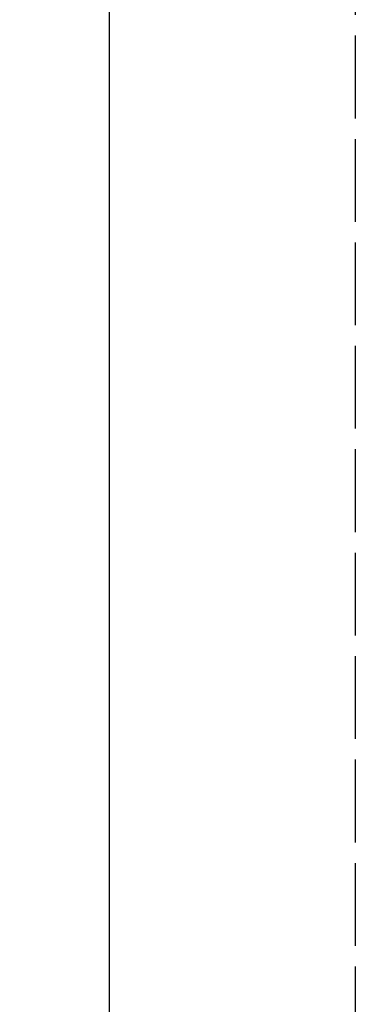
# Model space of a CAD drawing. Units: inches. Extents: x 1316 to 1777, y 813 to 1650.
# Tile 10 of 22: x 1316 to 1364, y 1434 to 1576. Entities that reach past the tile are written whole.
import ezdxf

# ---------------------------------------------------------------- set-up
doc = ezdxf.new("R2010")
doc.units = ezdxf.units.IN
doc.header["$MEASUREMENT"] = 0
doc.linetypes.add('ACAD_ISO02W100', pattern=[15, 12, -3])
doc.layers.add('A-ANNO-DIMS', color=2, linetype='Continuous', lineweight=18)
doc.layers.add('C-PROP', color=8, linetype='ACAD_ISO02W100', lineweight=25)
doc.styles.get("Standard").update_dxf_attribs({"font": 'arial.ttf'})
doc.dimstyles.get("Standard").update_dxf_attribs({"dimtxt": 7, "dimasz": 0.18, "dimexe": 0.18, "dimexo": 0.0625, "dimgap": 0.09, "dimtad": 0, "dimtih": 1, "dimtoh": 1, "dimzin": 0, "dimdsep": 46, "dimlunit": 3, "dimtxsty": 'Standard', "dimcen": 0.09, "dimadec": 0, "dimazin": 0, "dimtfac": 1, "dimtofl": 0, "dimtmove": 0, "dimatfit": 3, "dimfxl": 1, "dimtolj": 1, "dimtzin": 0, "dimarcsym": 0})

# ---------------------------------------------------------------- blocks, each defined once
blk = doc.blocks.new('*D23')
at = {"layer": 'A-ANNO-DIMS', "color": 0, "lineweight": -2, "transparency": 16777216}
for p, q in [((1328.47, 1604.17), (1328.87, 1604.17)), ((1328.69, 1603.99), (1328.69, 1282.59)), ((1328.69, 953.87), (1328.69, 1275.27)), ((1328.47, 953.69), (1328.87, 953.69))]:
    blk.add_line(p, q, dxfattribs=at)
at = {"layer": 'A-ANNO-DIMS', "color": 0, "transparency": 16777216}
for points in [[(1328.66, 1603.99), (1328.72, 1603.99), (1328.69, 1604.17)], [(1328.66, 953.87), (1328.72, 953.87), (1328.69, 953.69)]]:
    blk.add_solid(points, dxfattribs=at)
at = {"layer": 'Defpoints', "color": 0, "transparency": 16777216}
for p in [(1328.4, 1604.17), (1328.4, 953.69), (1328.69, 953.69)]:
    blk.add_point(p, dxfattribs=at)
at = {"layer": 'A-ANNO-DIMS', "color": 0, "transparency": 16777216, "insert": (1328.69, 1278.93), "char_height": 7, "width": 24.3281, "attachment_point": 5}
blk.add_mtext('\\A1;47\'-0"', dxfattribs=at)

msp = doc.modelspace()

# ---------------------------------------------------------------- linework, layer by layer
at = {"layer": 'C-PROP'}
msp.add_line((1364.399, 1604.173), (1364.399, 953.689), dxfattribs=at)

# ---------------------------------------------------------------- dimensions: what is measured, and where the dimension line sits
at = {"layer": 'A-ANNO-DIMS'}
dim = msp.add_linear_dim(base=(1328.686, 953.689), p1=(1328.404, 1604.173), p2=(1328.404, 953.689), angle=90, text='47\'-0"', dimstyle='Standard', override={"dimclrd": 0, "dimclre": 0, "dimclrt": 0}, dxfattribs=at)
dim.commit()
dim.dimension.update_dxf_attribs({"geometry": '*D23', "text_midpoint": (1328.686, 1278.931)})

doc.saveas('drawing.dxf')
